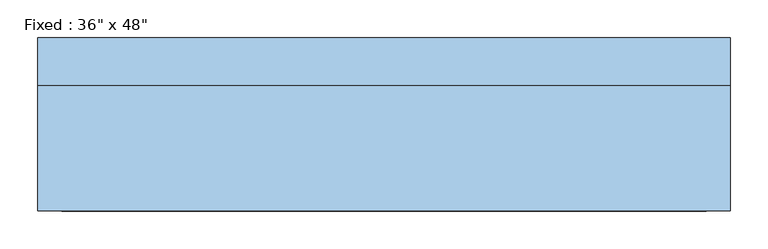
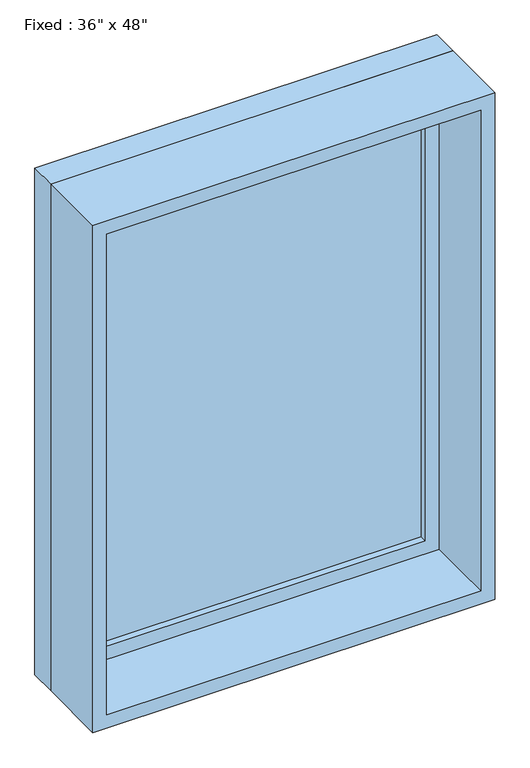
"""IFC4 building model written with IfcOpenShell, lengths in millimetres: window geometry."""

from ifc_helpers import new_model, si_unit, frame, origin, place, context, project, spatial, polyline, outline, extrude, source, transform, mapped, element, save


def window_c1f32544(model_context):
    return source(origin(), model_context, "Body", "SweptSolid", [
        extrude(outline(polyline([(355.6, 66.675), (-431.8, 66.675), (-431.8, 79.375), (355.6, 79.375), (355.6, 66.675)])), frame((0.0, 0.0, 977.9), z_axis=(0.0, 0.0, 1.0), x_axis=(1.0, 0.0, 0.0)), (0.0, 0.0, 1.0), 1092.2),
        extrude(outline(polyline([(2114.55, -476.25), (933.45, -476.25), (933.45, 400.05), (2114.55, 400.05), (2114.55, -476.25)]), holes=[polyline([(2070.1, -431.8), (2070.1, 355.6), (977.9, 355.6), (977.9, -431.8), (2070.1, -431.8)])]), frame((0.0, 50.8, 0.0), z_axis=(0.0, 1.0, 0.0), x_axis=(0.0, 0.0, 1.0)), (0.0, 0.0, 1.0), 44.45),
        extrude(outline(polyline([(2133.6, -495.3), (914.4, -495.3), (914.4, 419.1), (2133.6, 419.1), (2133.6, -495.3)]), holes=[polyline([(2101.85, -463.55), (2101.85, 387.35), (946.15, 387.35), (946.15, -463.55), (2101.85, -463.55)])]), frame((0.0, -114.3, 0.0), z_axis=(0.0, 1.0, 0.0), x_axis=(0.0, 0.0, 1.0)), (0.0, 0.0, 1.0), 165.1),
        extrude(outline(polyline([(2133.6, 419.1), (2133.6, -495.3), (914.4, -495.3), (914.4, 419.1), (2133.6, 419.1)]), holes=[polyline([(2114.55, 400.05), (933.45, 400.05), (933.45, -476.25), (2114.55, -476.25), (2114.55, 400.05)])]), frame((0.0, 50.8, 0.0), z_axis=(0.0, 1.0, 0.0), x_axis=(0.0, 0.0, 1.0)), (0.0, 0.0, 1.0), 63.5),
    ])


if __name__ == "__main__":
    model = new_model("IFC4")
    model_context = context("Model", 3, world=origin())
    ifc_project = project(units=[si_unit("LENGTHUNIT", "METRE", prefix="MILLI")], contexts=[model_context])
    site = spatial("IfcSite", under=ifc_project)
    building = spatial("IfcBuilding", under=site)
    placement = place(None, origin())
    window_shape = window_c1f32544(model_context)
    element("IfcWindow", 1, ObjectType="Fixed : 36\" x 48\"", at=placement, inside=building, context=model_context, shape_type="MappedRepresentation", body=[
        mapped(window_shape, transform((0.0, 0.0, 0.0), x_axis=(1.0, 0.0, 0.0), y_axis=(0.0, 1.0, 0.0), z_axis=(0.0, 0.0, 1.0))),
    ])
    save(model, "model.ifc")

# Revit data of these elements
# Type "Fixed : 36\" x 48\""
#   Type Mark = "W2"
#   Construction Type Id = "GSP4R"
#   Assembly Code = "B2020100"
#   Analytic Construction = "1/8 in Pilkington single glazing"
#   Visual Light Transmittance = 0.9
#   Solar Heat Gain Coefficient = 0.78
#   Heat Transfer Coefficient (U) = 0.6496 BTU/(h·ft²·°F)
#   Height = 4' - 0"
#   Default Sill Height = 3' - 0"
#   Width = 3' - 0"
#   Window Inset = 0' - 0 3/4"
#   Define Thermal Properties by = 1
#   Define Thermal Properties by = 1
#   Glass Pane Material = Glass
#   Sash Material = Sash
#   Wall Closure = (empty or 0)
# Element 1 (IfcWindow, "Fixed : 36\" x 48\"")
#   Materials on its faces: "Sash", "Glass"
# Materials
#   "Glass": class "Glass", colour RGB 0 128 192, transparency 0.75, Description = "Soda Lime Glass", Cost = 0
#   "Sash": class "Wood", colour RGB 224 178 126, transparency 0, Cost = 0
